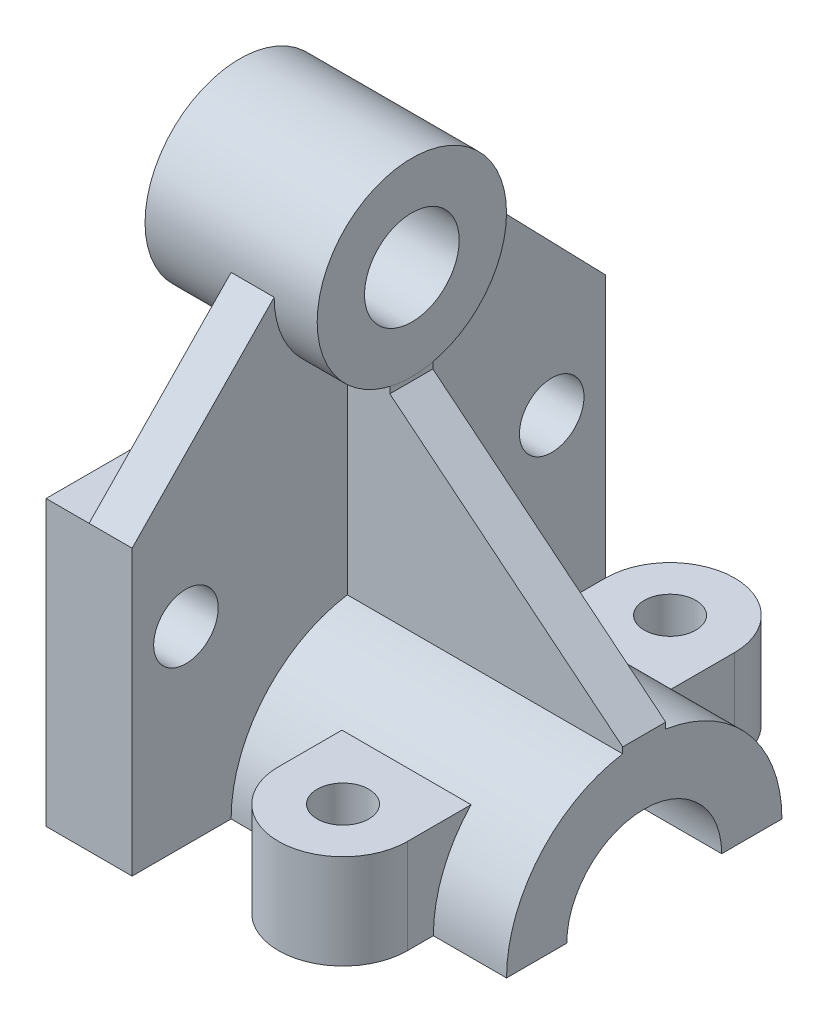
ISO-10303-21;
HEADER;
FILE_DESCRIPTION(('STEP AP214'),'2;1');
FILE_NAME('part.step','',(''),(''),'','','');
FILE_SCHEMA(('AUTOMOTIVE_DESIGN { 1 0 10303 214 1 1 1 1 }'));
ENDSEC;
DATA;
#1=APPLICATION_CONTEXT('core data for automotive mechanical design processes');
#2=APPLICATION_PROTOCOL_DEFINITION('international standard','automotive_design',2000,#1);
#3=PRODUCT_CONTEXT('',#1,'mechanical');
#4=PRODUCT('Part','Part','',(#3));
#5=PRODUCT_RELATED_PRODUCT_CATEGORY('part','',(#4));
#6=PRODUCT_DEFINITION_FORMATION('','',#4);
#7=PRODUCT_DEFINITION_CONTEXT('part definition',#1,'design');
#8=PRODUCT_DEFINITION('design','',#6,#7);
#9=PRODUCT_DEFINITION_SHAPE('','',#8);
#10=(LENGTH_UNIT() NAMED_UNIT(*) SI_UNIT(.MILLI.,.METRE.));
#11=(NAMED_UNIT(*) PLANE_ANGLE_UNIT() SI_UNIT($,.RADIAN.));
#12=(NAMED_UNIT(*) SI_UNIT($,.STERADIAN.) SOLID_ANGLE_UNIT());
#13=UNCERTAINTY_MEASURE_WITH_UNIT(LENGTH_MEASURE(1.E-05),#10,'distance_accuracy_value','');
#14=(GEOMETRIC_REPRESENTATION_CONTEXT(3) GLOBAL_UNCERTAINTY_ASSIGNED_CONTEXT((#13)) GLOBAL_UNIT_ASSIGNED_CONTEXT((#10,
#11,#12)) REPRESENTATION_CONTEXT('',''));
#15=CARTESIAN_POINT('',(0.,0.,0.));
#16=DIRECTION('',(0.,0.,1.));
#17=DIRECTION('',(1.,0.,0.));
#18=AXIS2_PLACEMENT_3D('',#15,#16,#17);
#19=CARTESIAN_POINT('',(10.,67.,0.));
#20=DIRECTION('',(1.,0.,0.));
#21=DIRECTION('',(0.,0.,-1.));
#22=AXIS2_PLACEMENT_3D('',#19,#20,#21);
#23=PLANE('',#22);
#24=CARTESIAN_POINT('',(10.,11.,-42.5));
#25=DIRECTION('',(1.,0.,0.));
#26=DIRECTION('',(0.,0.,-1.));
#27=AXIS2_PLACEMENT_3D('',#24,#25,#26);
#28=CIRCLE('',#27,7.5);
#29=CARTESIAN_POINT('',(10.,11.,-50.));
#30=VERTEX_POINT('',#29);
#31=EDGE_CURVE('E342',#30,#30,#28,.T.);
#32=ORIENTED_EDGE('',*,*,#31,.F.);
#33=EDGE_LOOP('',(#32));
#34=FACE_BOUND('',#33,.T.);
#35=DIRECTION('',(0.,-1.,0.));
#36=VECTOR('',#35,1.);
#37=CARTESIAN_POINT('',(10.,44.,-5.));
#38=LINE('',#37,#36);
#39=CARTESIAN_POINT('',(10.,45.5757147143715,-5.));
#40=VERTEX_POINT('',#39);
#41=CARTESIAN_POINT('',(10.,-1.39303874144178,-5.));
#42=VERTEX_POINT('',#41);
#43=EDGE_CURVE('E65',#40,#42,#38,.T.);
#44=ORIENTED_EDGE('',*,*,#43,.T.);
#45=CARTESIAN_POINT('',(10.,-33.,0.));
#46=DIRECTION('',(1.,0.,0.));
#47=DIRECTION('',(0.,0.,-1.));
#48=AXIS2_PLACEMENT_3D('',#45,#46,#47);
#49=CIRCLE('',#48,32.);
#50=CARTESIAN_POINT('',(10.,-33.,-32.));
#51=VERTEX_POINT('',#50);
#52=EDGE_CURVE('E314',#51,#42,#49,.T.);
#53=ORIENTED_EDGE('',*,*,#52,.F.);
#54=DIRECTION('',(0.,0.,-1.));
#55=VECTOR('',#54,1.);
#56=CARTESIAN_POINT('',(10.,-33.,55.));
#57=LINE('',#56,#55);
#58=CARTESIAN_POINT('',(10.,-33.,-55.));
#59=VERTEX_POINT('',#58);
#60=EDGE_CURVE('E354',#51,#59,#57,.T.);
#61=ORIENTED_EDGE('',*,*,#60,.T.);
#62=DIRECTION('',(0.,1.,0.));
#63=VECTOR('',#62,1.);
#64=CARTESIAN_POINT('',(10.,33.,-55.));
#65=LINE('',#64,#63);
#66=CARTESIAN_POINT('',(10.,33.,-55.));
#67=VERTEX_POINT('',#66);
#68=EDGE_CURVE('E350',#59,#67,#65,.T.);
#69=ORIENTED_EDGE('',*,*,#68,.T.);
#70=DIRECTION('',(0.,0.717580691628316,0.69647537716866));
#71=VECTOR('',#70,1.);
#72=CARTESIAN_POINT('',(10.,33.,-55.));
#73=LINE('',#72,#71);
#74=CARTESIAN_POINT('',(10.,67.,-22.));
#75=VERTEX_POINT('',#74);
#76=EDGE_CURVE('E391',#67,#75,#73,.T.);
#77=ORIENTED_EDGE('',*,*,#76,.T.);
#78=CARTESIAN_POINT('',(10.,67.,0.));
#79=DIRECTION('',(-1.,0.,0.));
#80=DIRECTION('',(0.,0.,-1.));
#81=AXIS2_PLACEMENT_3D('',#78,#79,#80);
#82=CIRCLE('',#81,22.);
#83=EDGE_CURVE('E414',#75,#40,#82,.T.);
#84=ORIENTED_EDGE('',*,*,#83,.T.);
#85=EDGE_LOOP('',(#44,#53,#61,#69,#77,#84));
#86=FACE_BOUND('',#85,.T.);
#87=ADVANCED_FACE('F39',(#34,#86),#23,.T.);
#88=CARTESIAN_POINT('',(10.,11.,42.5));
#89=DIRECTION('',(1.,0.,0.));
#90=DIRECTION('',(0.,0.,1.));
#91=AXIS2_PLACEMENT_3D('',#88,#89,#90);
#92=CIRCLE('',#91,7.5);
#93=CARTESIAN_POINT('',(10.,11.,50.));
#94=VERTEX_POINT('',#93);
#95=EDGE_CURVE('E341',#94,#94,#92,.T.);
#96=ORIENTED_EDGE('',*,*,#95,.F.);
#97=EDGE_LOOP('',(#96));
#98=FACE_BOUND('',#97,.T.);
#99=CARTESIAN_POINT('',(10.,-1.39303874144178,5.));
#100=VERTEX_POINT('',#99);
#101=CARTESIAN_POINT('',(10.,-33.,32.));
#102=VERTEX_POINT('',#101);
#103=EDGE_CURVE('E321',#100,#102,#49,.T.);
#104=ORIENTED_EDGE('',*,*,#103,.F.);
#105=DIRECTION('',(0.,-1.,0.));
#106=VECTOR('',#105,1.);
#107=CARTESIAN_POINT('',(10.,44.,5.));
#108=LINE('',#107,#106);
#109=CARTESIAN_POINT('',(10.,45.5757147143715,5.));
#110=VERTEX_POINT('',#109);
#111=EDGE_CURVE('E53',#110,#100,#108,.T.);
#112=ORIENTED_EDGE('',*,*,#111,.F.);
#113=CARTESIAN_POINT('',(10.,67.,22.));
#114=VERTEX_POINT('',#113);
#115=EDGE_CURVE('E413',#110,#114,#82,.T.);
#116=ORIENTED_EDGE('',*,*,#115,.T.);
#117=DIRECTION('',(0.,-0.717580691628316,0.69647537716866));
#118=VECTOR('',#117,1.);
#119=CARTESIAN_POINT('',(10.,67.,22.));
#120=LINE('',#119,#118);
#121=CARTESIAN_POINT('',(10.,33.,55.));
#122=VERTEX_POINT('',#121);
#123=EDGE_CURVE('E399',#114,#122,#120,.T.);
#124=ORIENTED_EDGE('',*,*,#123,.T.);
#125=DIRECTION('',(0.,-1.,0.));
#126=VECTOR('',#125,1.);
#127=CARTESIAN_POINT('',(10.,33.,55.));
#128=LINE('',#127,#126);
#129=CARTESIAN_POINT('',(10.,-33.,55.));
#130=VERTEX_POINT('',#129);
#131=EDGE_CURVE('E355',#122,#130,#128,.T.);
#132=ORIENTED_EDGE('',*,*,#131,.T.);
#133=EDGE_CURVE('E358',#130,#102,#57,.T.);
#134=ORIENTED_EDGE('',*,*,#133,.T.);
#135=EDGE_LOOP('',(#104,#112,#116,#124,#132,#134));
#136=FACE_BOUND('',#135,.T.);
#137=ADVANCED_FACE('F458',(#98,#136),#23,.T.);
#138=CARTESIAN_POINT('',(74.,-33.,0.));
#139=DIRECTION('',(-1.,0.,0.));
#140=DIRECTION('',(0.,0.,1.));
#141=AXIS2_PLACEMENT_3D('',#138,#139,#140);
#142=CYLINDRICAL_SURFACE('',#141,32.);
#143=DIRECTION('',(-1.,0.,0.));
#144=VECTOR('',#143,1.);
#145=CARTESIAN_POINT('',(74.,-1.39303874144178,-5.));
#146=LINE('',#145,#144);
#147=CARTESIAN_POINT('',(74.,-1.39303874144178,-5.));
#148=VERTEX_POINT('',#147);
#149=EDGE_CURVE('E238',#148,#42,#146,.T.);
#150=ORIENTED_EDGE('',*,*,#149,.F.);
#151=CARTESIAN_POINT('',(74.,-33.,0.));
#152=DIRECTION('',(1.,0.,0.));
#153=DIRECTION('',(0.,0.,-1.));
#154=AXIS2_PLACEMENT_3D('',#151,#152,#153);
#155=CIRCLE('',#154,32.);
#156=CARTESIAN_POINT('',(74.,-33.,-32.));
#157=VERTEX_POINT('',#156);
#158=EDGE_CURVE('E234',#157,#148,#155,.T.);
#159=ORIENTED_EDGE('',*,*,#158,.F.);
#160=DIRECTION('',(-1.,0.,0.));
#161=VECTOR('',#160,1.);
#162=CARTESIAN_POINT('',(74.,-33.,-32.));
#163=LINE('',#162,#161);
#164=CARTESIAN_POINT('',(57.,-33.,-32.));
#165=VERTEX_POINT('',#164);
#166=EDGE_CURVE('E335',#157,#165,#163,.T.);
#167=ORIENTED_EDGE('',*,*,#166,.T.);
#168=CARTESIAN_POINT('',(57.,-33.,0.));
#169=DIRECTION('',(1.,0.,0.));
#170=DIRECTION('',(0.,0.,-1.));
#171=AXIS2_PLACEMENT_3D('',#168,#169,#170);
#172=CIRCLE('',#171,32.);
#173=CARTESIAN_POINT('',(57.,-11.,-23.2379000772445));
#174=VERTEX_POINT('',#173);
#175=EDGE_CURVE('E382',#165,#174,#172,.T.);
#176=ORIENTED_EDGE('',*,*,#175,.T.);
#177=DIRECTION('',(-1.,0.,0.));
#178=VECTOR('',#177,1.);
#179=CARTESIAN_POINT('',(74.,-11.,-23.2379000772445));
#180=LINE('',#179,#178);
#181=CARTESIAN_POINT('',(27.,-11.,-23.2379000772445));
#182=VERTEX_POINT('',#181);
#183=EDGE_CURVE('E377',#182,#174,#180,.F.);
#184=ORIENTED_EDGE('',*,*,#183,.F.);
#185=CARTESIAN_POINT('',(27.,-33.,0.));
#186=DIRECTION('',(-1.,0.,0.));
#187=DIRECTION('',(0.,0.,1.));
#188=AXIS2_PLACEMENT_3D('',#185,#186,#187);
#189=CIRCLE('',#188,32.);
#190=CARTESIAN_POINT('',(27.,-33.,-32.));
#191=VERTEX_POINT('',#190);
#192=EDGE_CURVE('E384',#182,#191,#189,.T.);
#193=ORIENTED_EDGE('',*,*,#192,.T.);
#194=EDGE_CURVE('E331',#191,#51,#163,.T.);
#195=ORIENTED_EDGE('',*,*,#194,.T.);
#196=ORIENTED_EDGE('',*,*,#52,.T.);
#197=EDGE_LOOP('',(#150,#159,#167,#176,#184,#193,#195,#196));
#198=FACE_BOUND('',#197,.T.);
#199=ADVANCED_FACE('F463',(#198),#142,.T.);
#200=DIRECTION('',(-1.,0.,0.));
#201=VECTOR('',#200,1.);
#202=CARTESIAN_POINT('',(74.,-1.39303874144179,5.));
#203=LINE('',#202,#201);
#204=CARTESIAN_POINT('',(74.,-1.39303874144179,5.));
#205=VERTEX_POINT('',#204);
#206=EDGE_CURVE('E232',#100,#205,#203,.F.);
#207=ORIENTED_EDGE('',*,*,#206,.F.);
#208=ORIENTED_EDGE('',*,*,#103,.T.);
#209=DIRECTION('',(-1.,0.,0.));
#210=VECTOR('',#209,1.);
#211=CARTESIAN_POINT('',(74.,-33.,32.));
#212=LINE('',#211,#210);
#213=CARTESIAN_POINT('',(27.,-33.,32.));
#214=VERTEX_POINT('',#213);
#215=EDGE_CURVE('E329',#214,#102,#212,.T.);
#216=ORIENTED_EDGE('',*,*,#215,.F.);
#217=CARTESIAN_POINT('',(27.,-33.,0.));
#218=DIRECTION('',(-1.,0.,0.));
#219=DIRECTION('',(0.,0.,1.));
#220=AXIS2_PLACEMENT_3D('',#217,#218,#219);
#221=CIRCLE('',#220,32.);
#222=CARTESIAN_POINT('',(27.,-11.,23.2379000772445));
#223=VERTEX_POINT('',#222);
#224=EDGE_CURVE('E386',#214,#223,#221,.T.);
#225=ORIENTED_EDGE('',*,*,#224,.T.);
#226=DIRECTION('',(-1.,0.,0.));
#227=VECTOR('',#226,1.);
#228=CARTESIAN_POINT('',(74.,-11.,23.2379000772445));
#229=LINE('',#228,#227);
#230=CARTESIAN_POINT('',(57.,-11.,23.2379000772445));
#231=VERTEX_POINT('',#230);
#232=EDGE_CURVE('E387',#223,#231,#229,.F.);
#233=ORIENTED_EDGE('',*,*,#232,.T.);
#234=CARTESIAN_POINT('',(57.,-33.,0.));
#235=DIRECTION('',(1.,0.,0.));
#236=DIRECTION('',(0.,0.,-1.));
#237=AXIS2_PLACEMENT_3D('',#234,#235,#236);
#238=CIRCLE('',#237,32.);
#239=CARTESIAN_POINT('',(57.,-33.,32.));
#240=VERTEX_POINT('',#239);
#241=EDGE_CURVE('E394',#231,#240,#238,.T.);
#242=ORIENTED_EDGE('',*,*,#241,.T.);
#243=CARTESIAN_POINT('',(74.,-33.,32.));
#244=VERTEX_POINT('',#243);
#245=EDGE_CURVE('E327',#244,#240,#212,.T.);
#246=ORIENTED_EDGE('',*,*,#245,.F.);
#247=EDGE_CURVE('E320',#205,#244,#155,.T.);
#248=ORIENTED_EDGE('',*,*,#247,.F.);
#249=EDGE_LOOP('',(#207,#208,#216,#225,#233,#242,#246,#248));
#250=FACE_BOUND('',#249,.T.);
#251=ADVANCED_FACE('F516',(#250),#142,.T.);
#252=CARTESIAN_POINT('',(-20.,67.,0.));
#253=DIRECTION('',(1.,0.,0.));
#254=DIRECTION('',(0.,0.,-1.));
#255=AXIS2_PLACEMENT_3D('',#252,#253,#254);
#256=CYLINDRICAL_SURFACE('',#255,22.);
#257=CARTESIAN_POINT('',(-20.,67.,0.));
#258=DIRECTION('',(1.,0.,0.));
#259=DIRECTION('',(0.,0.,-1.));
#260=AXIS2_PLACEMENT_3D('',#257,#258,#259);
#261=CIRCLE('',#260,22.);
#262=CARTESIAN_POINT('',(-20.,67.,-22.));
#263=VERTEX_POINT('',#262);
#264=EDGE_CURVE('E11',#263,#263,#261,.T.);
#265=ORIENTED_EDGE('',*,*,#264,.T.);
#266=EDGE_LOOP('',(#265));
#267=FACE_BOUND('',#266,.T.);
#268=CARTESIAN_POINT('',(20.,67.,0.));
#269=DIRECTION('',(1.,0.,0.));
#270=DIRECTION('',(0.,0.,-1.));
#271=AXIS2_PLACEMENT_3D('',#268,#269,#270);
#272=CIRCLE('',#271,22.);
#273=CARTESIAN_POINT('',(20.,67.,-22.));
#274=VERTEX_POINT('',#273);
#275=EDGE_CURVE('E429',#274,#274,#272,.T.);
#276=ORIENTED_EDGE('',*,*,#275,.F.);
#277=EDGE_LOOP('',(#276));
#278=FACE_BOUND('',#277,.T.);
#279=CARTESIAN_POINT('',(19.8821035699118,67.,0.));
#280=DIRECTION('',(-1.,0.,0.));
#281=DIRECTION('',(0.,0.,1.));
#282=AXIS2_PLACEMENT_3D('',#279,#280,#281);
#283=CIRCLE('',#282,22.);
#284=CARTESIAN_POINT('',(19.8821035699118,45.5757147143715,5.));
#285=VERTEX_POINT('',#284);
#286=CARTESIAN_POINT('',(19.8821035699118,45.5757147143715,-5.));
#287=VERTEX_POINT('',#286);
#288=EDGE_CURVE('E255',#285,#287,#283,.F.);
#289=ORIENTED_EDGE('',*,*,#288,.T.);
#290=DIRECTION('',(1.,0.,0.));
#291=VECTOR('',#290,1.);
#292=CARTESIAN_POINT('',(-20.,45.5757147143715,-5.));
#293=LINE('',#292,#291);
#294=EDGE_CURVE('E248',#287,#40,#293,.F.);
#295=ORIENTED_EDGE('',*,*,#294,.T.);
#296=ORIENTED_EDGE('',*,*,#83,.F.);
#297=DIRECTION('',(1.,0.,0.));
#298=VECTOR('',#297,1.);
#299=CARTESIAN_POINT('',(0.,67.,-22.));
#300=LINE('',#299,#298);
#301=CARTESIAN_POINT('',(0.,67.,-22.));
#302=VERTEX_POINT('',#301);
#303=EDGE_CURVE('E422',#302,#75,#300,.T.);
#304=ORIENTED_EDGE('',*,*,#303,.F.);
#305=CARTESIAN_POINT('',(0.,67.,0.));
#306=DIRECTION('',(-1.,0.,0.));
#307=DIRECTION('',(0.,0.,-1.));
#308=AXIS2_PLACEMENT_3D('',#305,#306,#307);
#309=CIRCLE('',#308,22.);
#310=CARTESIAN_POINT('',(0.,67.,22.));
#311=VERTEX_POINT('',#310);
#312=EDGE_CURVE('E401',#302,#311,#309,.T.);
#313=ORIENTED_EDGE('',*,*,#312,.T.);
#314=DIRECTION('',(1.,0.,0.));
#315=VECTOR('',#314,1.);
#316=CARTESIAN_POINT('',(0.,67.,22.));
#317=LINE('',#316,#315);
#318=EDGE_CURVE('E417',#311,#114,#317,.T.);
#319=ORIENTED_EDGE('',*,*,#318,.T.);
#320=ORIENTED_EDGE('',*,*,#115,.F.);
#321=DIRECTION('',(1.,0.,0.));
#322=VECTOR('',#321,1.);
#323=CARTESIAN_POINT('',(-20.,45.5757147143715,5.));
#324=LINE('',#323,#322);
#325=EDGE_CURVE('E250',#110,#285,#324,.T.);
#326=ORIENTED_EDGE('',*,*,#325,.T.);
#327=EDGE_LOOP('',(#289,#295,#296,#304,#313,#319,#320,#326));
#328=FACE_BOUND('',#327,.T.);
#329=ADVANCED_FACE('F41',(#267,#278,#328),#256,.T.);
#330=CARTESIAN_POINT('',(-20.,67.,0.));
#331=DIRECTION('',(1.,0.,0.));
#332=DIRECTION('',(0.,0.,-1.));
#333=AXIS2_PLACEMENT_3D('',#330,#331,#332);
#334=PLANE('',#333);
#335=CARTESIAN_POINT('',(-20.,67.,0.));
#336=DIRECTION('',(1.,0.,0.));
#337=DIRECTION('',(0.,0.,-1.));
#338=AXIS2_PLACEMENT_3D('',#335,#336,#337);
#339=CIRCLE('',#338,11.);
#340=CARTESIAN_POINT('',(-20.,67.,-11.));
#341=VERTEX_POINT('',#340);
#342=EDGE_CURVE('E50',#341,#341,#339,.T.);
#343=ORIENTED_EDGE('',*,*,#342,.T.);
#344=EDGE_LOOP('',(#343));
#345=FACE_BOUND('',#344,.T.);
#346=ORIENTED_EDGE('',*,*,#264,.F.);
#347=EDGE_LOOP('',(#346));
#348=FACE_BOUND('',#347,.T.);
#349=ADVANCED_FACE('F432',(#345,#348),#334,.F.);
#350=CARTESIAN_POINT('',(-20.,67.,0.));
#351=DIRECTION('',(1.,0.,0.));
#352=DIRECTION('',(0.,0.,-1.));
#353=AXIS2_PLACEMENT_3D('',#350,#351,#352);
#354=CYLINDRICAL_SURFACE('',#353,11.);
#355=ORIENTED_EDGE('',*,*,#342,.F.);
#356=EDGE_LOOP('',(#355));
#357=FACE_BOUND('',#356,.T.);
#358=CARTESIAN_POINT('',(20.,67.,0.));
#359=DIRECTION('',(1.,0.,0.));
#360=DIRECTION('',(0.,0.,-1.));
#361=AXIS2_PLACEMENT_3D('',#358,#359,#360);
#362=CIRCLE('',#361,11.);
#363=CARTESIAN_POINT('',(20.,67.,-11.));
#364=VERTEX_POINT('',#363);
#365=EDGE_CURVE('E418',#364,#364,#362,.T.);
#366=ORIENTED_EDGE('',*,*,#365,.T.);
#367=EDGE_LOOP('',(#366));
#368=FACE_BOUND('',#367,.T.);
#369=ADVANCED_FACE('F440',(#357,#368),#354,.F.);
#370=CARTESIAN_POINT('',(20.,67.,0.));
#371=DIRECTION('',(1.,0.,0.));
#372=DIRECTION('',(0.,0.,-1.));
#373=AXIS2_PLACEMENT_3D('',#370,#371,#372);
#374=PLANE('',#373);
#375=ORIENTED_EDGE('',*,*,#275,.T.);
#376=EDGE_LOOP('',(#375));
#377=FACE_BOUND('',#376,.T.);
#378=ORIENTED_EDGE('',*,*,#365,.F.);
#379=EDGE_LOOP('',(#378));
#380=FACE_BOUND('',#379,.T.);
#381=ADVANCED_FACE('F439',(#377,#380),#374,.T.);
#382=CARTESIAN_POINT('',(0.,67.,22.));
#383=DIRECTION('',(0.,0.69647537716866,0.717580691628316));
#384=DIRECTION('',(0.,-0.717580691628316,0.69647537716866));
#385=AXIS2_PLACEMENT_3D('',#382,#383,#384);
#386=PLANE('',#385);
#387=ORIENTED_EDGE('',*,*,#123,.F.);
#388=ORIENTED_EDGE('',*,*,#318,.F.);
#389=DIRECTION('',(0.,-0.717580691628316,0.69647537716866));
#390=VECTOR('',#389,1.);
#391=CARTESIAN_POINT('',(0.,67.,22.));
#392=LINE('',#391,#390);
#393=CARTESIAN_POINT('',(0.,33.,55.));
#394=VERTEX_POINT('',#393);
#395=EDGE_CURVE('E403',#311,#394,#392,.T.);
#396=ORIENTED_EDGE('',*,*,#395,.T.);
#397=DIRECTION('',(1.,0.,0.));
#398=VECTOR('',#397,1.);
#399=CARTESIAN_POINT('',(0.,33.,55.));
#400=LINE('',#399,#398);
#401=EDGE_CURVE('E416',#394,#122,#400,.T.);
#402=ORIENTED_EDGE('',*,*,#401,.T.);
#403=EDGE_LOOP('',(#387,#388,#396,#402));
#404=FACE_BOUND('',#403,.T.);
#405=ADVANCED_FACE('F444',(#404),#386,.T.);
#406=CARTESIAN_POINT('',(0.,33.,-55.));
#407=DIRECTION('',(0.,0.69647537716866,-0.717580691628316));
#408=DIRECTION('',(0.,0.717580691628316,0.69647537716866));
#409=AXIS2_PLACEMENT_3D('',#406,#407,#408);
#410=PLANE('',#409);
#411=ORIENTED_EDGE('',*,*,#76,.F.);
#412=DIRECTION('',(1.,0.,0.));
#413=VECTOR('',#412,1.);
#414=CARTESIAN_POINT('',(0.,33.,-55.));
#415=LINE('',#414,#413);
#416=CARTESIAN_POINT('',(0.,33.,-55.));
#417=VERTEX_POINT('',#416);
#418=EDGE_CURVE('E409',#417,#67,#415,.T.);
#419=ORIENTED_EDGE('',*,*,#418,.F.);
#420=DIRECTION('',(0.,0.717580691628316,0.69647537716866));
#421=VECTOR('',#420,1.);
#422=CARTESIAN_POINT('',(0.,33.,-55.));
#423=LINE('',#422,#421);
#424=EDGE_CURVE('E397',#417,#302,#423,.T.);
#425=ORIENTED_EDGE('',*,*,#424,.T.);
#426=ORIENTED_EDGE('',*,*,#303,.T.);
#427=EDGE_LOOP('',(#411,#419,#425,#426));
#428=FACE_BOUND('',#427,.T.);
#429=ADVANCED_FACE('F452',(#428),#410,.T.);
#430=CARTESIAN_POINT('',(0.,67.,0.));
#431=DIRECTION('',(1.,0.,0.));
#432=DIRECTION('',(0.,0.,-1.));
#433=AXIS2_PLACEMENT_3D('',#430,#431,#432);
#434=PLANE('',#433);
#435=DIRECTION('',(0.,0.,-1.));
#436=VECTOR('',#435,1.);
#437=CARTESIAN_POINT('',(0.,33.,-55.));
#438=LINE('',#437,#436);
#439=EDGE_CURVE('E396',#394,#417,#438,.T.);
#440=ORIENTED_EDGE('',*,*,#439,.F.);
#441=ORIENTED_EDGE('',*,*,#395,.F.);
#442=ORIENTED_EDGE('',*,*,#312,.F.);
#443=ORIENTED_EDGE('',*,*,#424,.F.);
#444=EDGE_LOOP('',(#440,#441,#442,#443));
#445=FACE_BOUND('',#444,.T.);
#446=ADVANCED_FACE('F470',(#445),#434,.F.);
#447=CARTESIAN_POINT('',(10.,33.,55.));
#448=DIRECTION('',(0.,-1.,0.));
#449=DIRECTION('',(0.,0.,-1.));
#450=AXIS2_PLACEMENT_3D('',#447,#448,#449);
#451=PLANE('',#450);
#452=DIRECTION('',(-1.,0.,0.));
#453=VECTOR('',#452,1.);
#454=CARTESIAN_POINT('',(10.,33.,55.));
#455=LINE('',#454,#453);
#456=CARTESIAN_POINT('',(-10.,33.,55.));
#457=VERTEX_POINT('',#456);
#458=EDGE_CURVE('E372',#394,#457,#455,.T.);
#459=ORIENTED_EDGE('',*,*,#458,.F.);
#460=ORIENTED_EDGE('',*,*,#439,.T.);
#461=DIRECTION('',(-1.,0.,0.));
#462=VECTOR('',#461,1.);
#463=CARTESIAN_POINT('',(10.,33.,-55.));
#464=LINE('',#463,#462);
#465=CARTESIAN_POINT('',(-10.,33.,-55.));
#466=VERTEX_POINT('',#465);
#467=EDGE_CURVE('E376',#417,#466,#464,.T.);
#468=ORIENTED_EDGE('',*,*,#467,.T.);
#469=DIRECTION('',(0.,0.,1.));
#470=VECTOR('',#469,1.);
#471=CARTESIAN_POINT('',(-10.,33.,55.));
#472=LINE('',#471,#470);
#473=EDGE_CURVE('E361',#466,#457,#472,.T.);
#474=ORIENTED_EDGE('',*,*,#473,.T.);
#475=EDGE_LOOP('',(#459,#460,#468,#474));
#476=FACE_BOUND('',#475,.T.);
#477=ADVANCED_FACE('F471',(#476),#451,.F.);
#478=CARTESIAN_POINT('',(10.,0.,0.));
#479=DIRECTION('',(1.,0.,0.));
#480=DIRECTION('',(0.,0.,-1.));
#481=AXIS2_PLACEMENT_3D('',#478,#479,#480);
#482=PLANE('',#481);
#483=CARTESIAN_POINT('',(10.,-33.,0.));
#484=DIRECTION('',(-1.,0.,0.));
#485=DIRECTION('',(0.,0.,-1.));
#486=AXIS2_PLACEMENT_3D('',#483,#484,#485);
#487=CIRCLE('',#486,18.);
#488=CARTESIAN_POINT('',(10.,-33.,18.));
#489=VERTEX_POINT('',#488);
#490=CARTESIAN_POINT('',(10.,-33.,-18.));
#491=VERTEX_POINT('',#490);
#492=EDGE_CURVE('E307',#489,#491,#487,.T.);
#493=ORIENTED_EDGE('',*,*,#492,.F.);
#494=EDGE_CURVE('E359',#489,#491,#57,.T.);
#495=ORIENTED_EDGE('',*,*,#494,.T.);
#496=EDGE_LOOP('',(#493,#495));
#497=FACE_BOUND('',#496,.T.);
#498=ADVANCED_FACE('F532',(#497),#482,.T.);
#499=CARTESIAN_POINT('',(10.,33.,-55.));
#500=DIRECTION('',(0.,0.,1.));
#501=DIRECTION('',(0.,-1.,0.));
#502=AXIS2_PLACEMENT_3D('',#499,#500,#501);
#503=PLANE('',#502);
#504=DIRECTION('',(0.,1.,0.));
#505=VECTOR('',#504,1.);
#506=CARTESIAN_POINT('',(-10.,33.,-55.));
#507=LINE('',#506,#505);
#508=CARTESIAN_POINT('',(-10.,-33.,-55.));
#509=VERTEX_POINT('',#508);
#510=EDGE_CURVE('E338',#509,#466,#507,.T.);
#511=ORIENTED_EDGE('',*,*,#510,.T.);
#512=ORIENTED_EDGE('',*,*,#467,.F.);
#513=ORIENTED_EDGE('',*,*,#418,.T.);
#514=ORIENTED_EDGE('',*,*,#68,.F.);
#515=DIRECTION('',(-1.,0.,0.));
#516=VECTOR('',#515,1.);
#517=CARTESIAN_POINT('',(10.,-33.,-55.));
#518=LINE('',#517,#516);
#519=EDGE_CURVE('E360',#59,#509,#518,.T.);
#520=ORIENTED_EDGE('',*,*,#519,.T.);
#521=EDGE_LOOP('',(#511,#512,#513,#514,#520));
#522=FACE_BOUND('',#521,.T.);
#523=ADVANCED_FACE('F485',(#522),#503,.F.);
#524=CARTESIAN_POINT('',(10.,33.,55.));
#525=DIRECTION('',(0.,0.,-1.));
#526=DIRECTION('',(0.,1.,0.));
#527=AXIS2_PLACEMENT_3D('',#524,#525,#526);
#528=PLANE('',#527);
#529=DIRECTION('',(0.,-1.,0.));
#530=VECTOR('',#529,1.);
#531=CARTESIAN_POINT('',(-10.,33.,55.));
#532=LINE('',#531,#530);
#533=CARTESIAN_POINT('',(-10.,-33.,55.));
#534=VERTEX_POINT('',#533);
#535=EDGE_CURVE('E366',#457,#534,#532,.T.);
#536=ORIENTED_EDGE('',*,*,#535,.T.);
#537=DIRECTION('',(-1.,0.,0.));
#538=VECTOR('',#537,1.);
#539=CARTESIAN_POINT('',(10.,-33.,55.));
#540=LINE('',#539,#538);
#541=EDGE_CURVE('E371',#130,#534,#540,.T.);
#542=ORIENTED_EDGE('',*,*,#541,.F.);
#543=ORIENTED_EDGE('',*,*,#131,.F.);
#544=ORIENTED_EDGE('',*,*,#401,.F.);
#545=ORIENTED_EDGE('',*,*,#458,.T.);
#546=EDGE_LOOP('',(#536,#542,#543,#544,#545));
#547=FACE_BOUND('',#546,.T.);
#548=ADVANCED_FACE('F491',(#547),#528,.F.);
#549=CARTESIAN_POINT('',(10.,-33.,55.));
#550=DIRECTION('',(0.,1.,0.));
#551=DIRECTION('',(0.,0.,1.));
#552=AXIS2_PLACEMENT_3D('',#549,#550,#551);
#553=PLANE('',#552);
#554=CARTESIAN_POINT('',(42.,-33.,-38.));
#555=DIRECTION('',(0.,1.,0.));
#556=DIRECTION('',(0.,0.,1.));
#557=AXIS2_PLACEMENT_3D('',#554,#555,#556);
#558=CIRCLE('',#557,6.);
#559=CARTESIAN_POINT('',(42.,-33.,-32.));
#560=VERTEX_POINT('',#559);
#561=EDGE_CURVE('E259',#560,#560,#558,.T.);
#562=ORIENTED_EDGE('',*,*,#561,.T.);
#563=EDGE_LOOP('',(#562));
#564=FACE_BOUND('',#563,.T.);
#565=CARTESIAN_POINT('',(42.,-33.,38.));
#566=DIRECTION('',(0.,1.,0.));
#567=DIRECTION('',(0.,0.,1.));
#568=AXIS2_PLACEMENT_3D('',#565,#566,#567);
#569=CIRCLE('',#568,6.);
#570=CARTESIAN_POINT('',(42.,-33.,44.));
#571=VERTEX_POINT('',#570);
#572=EDGE_CURVE('E226',#571,#571,#569,.T.);
#573=ORIENTED_EDGE('',*,*,#572,.T.);
#574=EDGE_LOOP('',(#573));
#575=FACE_BOUND('',#574,.T.);
#576=ORIENTED_EDGE('',*,*,#494,.F.);
#577=DIRECTION('',(-1.,0.,0.));
#578=VECTOR('',#577,1.);
#579=CARTESIAN_POINT('',(74.,-33.,18.));
#580=LINE('',#579,#578);
#581=CARTESIAN_POINT('',(74.,-33.,18.));
#582=VERTEX_POINT('',#581);
#583=EDGE_CURVE('E322',#582,#489,#580,.T.);
#584=ORIENTED_EDGE('',*,*,#583,.F.);
#585=DIRECTION('',(0.,0.,-1.));
#586=VECTOR('',#585,1.);
#587=CARTESIAN_POINT('',(74.,-33.,32.));
#588=LINE('',#587,#586);
#589=EDGE_CURVE('E316',#244,#582,#588,.T.);
#590=ORIENTED_EDGE('',*,*,#589,.F.);
#591=ORIENTED_EDGE('',*,*,#245,.T.);
#592=DIRECTION('',(0.,0.,1.));
#593=VECTOR('',#592,1.);
#594=CARTESIAN_POINT('',(57.,-33.,18.));
#595=LINE('',#594,#593);
#596=CARTESIAN_POINT('',(57.,-33.,38.));
#597=VERTEX_POINT('',#596);
#598=EDGE_CURVE('E273',#240,#597,#595,.T.);
#599=ORIENTED_EDGE('',*,*,#598,.T.);
#600=CARTESIAN_POINT('',(42.,-33.,38.));
#601=DIRECTION('',(0.,-1.,0.));
#602=DIRECTION('',(0.,0.,1.));
#603=AXIS2_PLACEMENT_3D('',#600,#601,#602);
#604=CIRCLE('',#603,15.);
#605=CARTESIAN_POINT('',(27.,-33.,38.));
#606=VERTEX_POINT('',#605);
#607=EDGE_CURVE('E278',#597,#606,#604,.T.);
#608=ORIENTED_EDGE('',*,*,#607,.T.);
#609=DIRECTION('',(0.,0.,-1.));
#610=VECTOR('',#609,1.);
#611=CARTESIAN_POINT('',(27.,-33.,38.));
#612=LINE('',#611,#610);
#613=EDGE_CURVE('E280',#606,#214,#612,.T.);
#614=ORIENTED_EDGE('',*,*,#613,.T.);
#615=ORIENTED_EDGE('',*,*,#215,.T.);
#616=ORIENTED_EDGE('',*,*,#133,.F.);
#617=ORIENTED_EDGE('',*,*,#541,.T.);
#618=DIRECTION('',(0.,0.,-1.));
#619=VECTOR('',#618,1.);
#620=CARTESIAN_POINT('',(-10.,-33.,55.));
#621=LINE('',#620,#619);
#622=EDGE_CURVE('E353',#534,#509,#621,.T.);
#623=ORIENTED_EDGE('',*,*,#622,.T.);
#624=ORIENTED_EDGE('',*,*,#519,.F.);
#625=ORIENTED_EDGE('',*,*,#60,.F.);
#626=ORIENTED_EDGE('',*,*,#194,.F.);
#627=DIRECTION('',(0.,0.,-1.));
#628=VECTOR('',#627,1.);
#629=CARTESIAN_POINT('',(27.,-33.,-38.));
#630=LINE('',#629,#628);
#631=CARTESIAN_POINT('',(27.,-33.,-38.));
#632=VERTEX_POINT('',#631);
#633=EDGE_CURVE('E295',#191,#632,#630,.T.);
#634=ORIENTED_EDGE('',*,*,#633,.T.);
#635=CARTESIAN_POINT('',(42.,-33.,-38.));
#636=DIRECTION('',(0.,-1.,0.));
#637=DIRECTION('',(0.,0.,-1.));
#638=AXIS2_PLACEMENT_3D('',#635,#636,#637);
#639=CIRCLE('',#638,15.);
#640=CARTESIAN_POINT('',(57.,-33.,-38.));
#641=VERTEX_POINT('',#640);
#642=EDGE_CURVE('E282',#632,#641,#639,.T.);
#643=ORIENTED_EDGE('',*,*,#642,.T.);
#644=DIRECTION('',(0.,0.,1.));
#645=VECTOR('',#644,1.);
#646=CARTESIAN_POINT('',(57.,-33.,-18.));
#647=LINE('',#646,#645);
#648=EDGE_CURVE('E305',#641,#165,#647,.T.);
#649=ORIENTED_EDGE('',*,*,#648,.T.);
#650=ORIENTED_EDGE('',*,*,#166,.F.);
#651=DIRECTION('',(0.,0.,-1.));
#652=VECTOR('',#651,1.);
#653=CARTESIAN_POINT('',(74.,-33.,-18.));
#654=LINE('',#653,#652);
#655=CARTESIAN_POINT('',(74.,-33.,-18.));
#656=VERTEX_POINT('',#655);
#657=EDGE_CURVE('E313',#656,#157,#654,.T.);
#658=ORIENTED_EDGE('',*,*,#657,.F.);
#659=DIRECTION('',(-1.,0.,0.));
#660=VECTOR('',#659,1.);
#661=CARTESIAN_POINT('',(74.,-33.,-18.));
#662=LINE('',#661,#660);
#663=EDGE_CURVE('E332',#656,#491,#662,.T.);
#664=ORIENTED_EDGE('',*,*,#663,.T.);
#665=EDGE_LOOP('',(#576,#584,#590,#591,#599,#608,#614,#615,#616,#617,#623,#624,#625,#626,#634,
#643,#649,#650,#658,#664));
#666=FACE_BOUND('',#665,.T.);
#667=ADVANCED_FACE('F497',(#564,#575,#666),#553,.F.);
#668=CARTESIAN_POINT('',(-10.,0.,0.));
#669=DIRECTION('',(1.,0.,0.));
#670=DIRECTION('',(0.,0.,-1.));
#671=AXIS2_PLACEMENT_3D('',#668,#669,#670);
#672=PLANE('',#671);
#673=CARTESIAN_POINT('',(-10.,11.,-42.5));
#674=DIRECTION('',(1.,0.,0.));
#675=DIRECTION('',(0.,0.,-1.));
#676=AXIS2_PLACEMENT_3D('',#673,#674,#675);
#677=CIRCLE('',#676,7.5);
#678=CARTESIAN_POINT('',(-10.,11.,-50.));
#679=VERTEX_POINT('',#678);
#680=EDGE_CURVE('E340',#679,#679,#677,.T.);
#681=ORIENTED_EDGE('',*,*,#680,.T.);
#682=EDGE_LOOP('',(#681));
#683=FACE_BOUND('',#682,.T.);
#684=CARTESIAN_POINT('',(-10.,11.,42.5));
#685=DIRECTION('',(1.,0.,0.));
#686=DIRECTION('',(0.,0.,1.));
#687=AXIS2_PLACEMENT_3D('',#684,#685,#686);
#688=CIRCLE('',#687,7.5);
#689=CARTESIAN_POINT('',(-10.,11.,50.));
#690=VERTEX_POINT('',#689);
#691=EDGE_CURVE('E337',#690,#690,#688,.T.);
#692=ORIENTED_EDGE('',*,*,#691,.T.);
#693=EDGE_LOOP('',(#692));
#694=FACE_BOUND('',#693,.T.);
#695=ORIENTED_EDGE('',*,*,#510,.F.);
#696=ORIENTED_EDGE('',*,*,#622,.F.);
#697=ORIENTED_EDGE('',*,*,#535,.F.);
#698=ORIENTED_EDGE('',*,*,#473,.F.);
#699=EDGE_LOOP('',(#695,#696,#697,#698));
#700=FACE_BOUND('',#699,.T.);
#701=ADVANCED_FACE('F490',(#683,#694,#700),#672,.F.);
#702=CARTESIAN_POINT('',(-10.,11.,42.5));
#703=DIRECTION('',(1.,0.,0.));
#704=DIRECTION('',(0.,0.,-1.));
#705=AXIS2_PLACEMENT_3D('',#702,#703,#704);
#706=CYLINDRICAL_SURFACE('',#705,7.5);
#707=ORIENTED_EDGE('',*,*,#691,.F.);
#708=EDGE_LOOP('',(#707));
#709=FACE_BOUND('',#708,.T.);
#710=ORIENTED_EDGE('',*,*,#95,.T.);
#711=EDGE_LOOP('',(#710));
#712=FACE_BOUND('',#711,.T.);
#713=ADVANCED_FACE('F543',(#709,#712),#706,.F.);
#714=CARTESIAN_POINT('',(-10.,11.,-42.5));
#715=DIRECTION('',(1.,0.,0.));
#716=DIRECTION('',(0.,0.,-1.));
#717=AXIS2_PLACEMENT_3D('',#714,#715,#716);
#718=CYLINDRICAL_SURFACE('',#717,7.5);
#719=ORIENTED_EDGE('',*,*,#680,.F.);
#720=EDGE_LOOP('',(#719));
#721=FACE_BOUND('',#720,.T.);
#722=ORIENTED_EDGE('',*,*,#31,.T.);
#723=EDGE_LOOP('',(#722));
#724=FACE_BOUND('',#723,.T.);
#725=ADVANCED_FACE('F568',(#721,#724),#718,.F.);
#726=CARTESIAN_POINT('',(74.,-33.,0.));
#727=DIRECTION('',(-1.,0.,0.));
#728=DIRECTION('',(0.,0.,1.));
#729=AXIS2_PLACEMENT_3D('',#726,#727,#728);
#730=CYLINDRICAL_SURFACE('',#729,18.);
#731=ORIENTED_EDGE('',*,*,#492,.T.);
#732=ORIENTED_EDGE('',*,*,#663,.F.);
#733=CARTESIAN_POINT('',(74.,-33.,0.));
#734=DIRECTION('',(-1.,0.,0.));
#735=DIRECTION('',(0.,0.,-1.));
#736=AXIS2_PLACEMENT_3D('',#733,#734,#735);
#737=CIRCLE('',#736,18.);
#738=EDGE_CURVE('E311',#582,#656,#737,.T.);
#739=ORIENTED_EDGE('',*,*,#738,.F.);
#740=ORIENTED_EDGE('',*,*,#583,.T.);
#741=EDGE_LOOP('',(#731,#732,#739,#740));
#742=FACE_BOUND('',#741,.T.);
#743=ADVANCED_FACE('F521',(#742),#730,.F.);
#744=CARTESIAN_POINT('',(74.,-33.,0.));
#745=DIRECTION('',(1.,0.,0.));
#746=DIRECTION('',(0.,0.,-1.));
#747=AXIS2_PLACEMENT_3D('',#744,#745,#746);
#748=PLANE('',#747);
#749=ORIENTED_EDGE('',*,*,#158,.T.);
#750=DIRECTION('',(0.,1.,0.));
#751=VECTOR('',#750,1.);
#752=CARTESIAN_POINT('',(74.,-2.,-5.));
#753=LINE('',#752,#751);
#754=CARTESIAN_POINT('',(74.,0.,-5.));
#755=VERTEX_POINT('',#754);
#756=EDGE_CURVE('E214',#148,#755,#753,.T.);
#757=ORIENTED_EDGE('',*,*,#756,.T.);
#758=DIRECTION('',(0.,0.,-1.));
#759=VECTOR('',#758,1.);
#760=CARTESIAN_POINT('',(74.,0.,5.));
#761=LINE('',#760,#759);
#762=CARTESIAN_POINT('',(74.,0.,5.));
#763=VERTEX_POINT('',#762);
#764=EDGE_CURVE('E225',#763,#755,#761,.T.);
#765=ORIENTED_EDGE('',*,*,#764,.F.);
#766=DIRECTION('',(0.,1.,0.));
#767=VECTOR('',#766,1.);
#768=CARTESIAN_POINT('',(74.,-2.,5.));
#769=LINE('',#768,#767);
#770=EDGE_CURVE('E236',#205,#763,#769,.T.);
#771=ORIENTED_EDGE('',*,*,#770,.F.);
#772=ORIENTED_EDGE('',*,*,#247,.T.);
#773=ORIENTED_EDGE('',*,*,#589,.T.);
#774=ORIENTED_EDGE('',*,*,#738,.T.);
#775=ORIENTED_EDGE('',*,*,#657,.T.);
#776=EDGE_LOOP('',(#749,#757,#765,#771,#772,#773,#774,#775));
#777=FACE_BOUND('',#776,.T.);
#778=ADVANCED_FACE('F235',(#777),#748,.T.);
#779=CARTESIAN_POINT('',(42.,-11.,-38.));
#780=DIRECTION('',(0.,-1.,0.));
#781=DIRECTION('',(0.,0.,-1.));
#782=AXIS2_PLACEMENT_3D('',#779,#780,#781);
#783=PLANE('',#782);
#784=CARTESIAN_POINT('',(42.,-11.,-38.));
#785=DIRECTION('',(0.,1.,0.));
#786=DIRECTION('',(0.,0.,1.));
#787=AXIS2_PLACEMENT_3D('',#784,#785,#786);
#788=CIRCLE('',#787,6.);
#789=CARTESIAN_POINT('',(42.,-11.,-32.));
#790=VERTEX_POINT('',#789);
#791=EDGE_CURVE('E264',#790,#790,#788,.T.);
#792=ORIENTED_EDGE('',*,*,#791,.F.);
#793=EDGE_LOOP('',(#792));
#794=FACE_BOUND('',#793,.T.);
#795=DIRECTION('',(0.,0.,-1.));
#796=VECTOR('',#795,1.);
#797=CARTESIAN_POINT('',(27.,-11.,-38.));
#798=LINE('',#797,#796);
#799=CARTESIAN_POINT('',(27.,-11.,-38.));
#800=VERTEX_POINT('',#799);
#801=EDGE_CURVE('E300',#182,#800,#798,.T.);
#802=ORIENTED_EDGE('',*,*,#801,.F.);
#803=ORIENTED_EDGE('',*,*,#183,.T.);
#804=DIRECTION('',(0.,0.,1.));
#805=VECTOR('',#804,1.);
#806=CARTESIAN_POINT('',(57.,-11.,-18.));
#807=LINE('',#806,#805);
#808=CARTESIAN_POINT('',(57.,-11.,-38.));
#809=VERTEX_POINT('',#808);
#810=EDGE_CURVE('E291',#809,#174,#807,.T.);
#811=ORIENTED_EDGE('',*,*,#810,.F.);
#812=CARTESIAN_POINT('',(42.,-11.,-38.));
#813=DIRECTION('',(0.,-1.,0.));
#814=DIRECTION('',(0.,0.,-1.));
#815=AXIS2_PLACEMENT_3D('',#812,#813,#814);
#816=CIRCLE('',#815,15.);
#817=EDGE_CURVE('E289',#800,#809,#816,.T.);
#818=ORIENTED_EDGE('',*,*,#817,.F.);
#819=EDGE_LOOP('',(#802,#803,#811,#818));
#820=FACE_BOUND('',#819,.T.);
#821=ADVANCED_FACE('F583',(#794,#820),#783,.F.);
#822=CARTESIAN_POINT('',(42.,-11.,-38.));
#823=DIRECTION('',(0.,-1.,0.));
#824=DIRECTION('',(0.,0.,-1.));
#825=AXIS2_PLACEMENT_3D('',#822,#823,#824);
#826=CYLINDRICAL_SURFACE('',#825,15.);
#827=ORIENTED_EDGE('',*,*,#642,.F.);
#828=DIRECTION('',(0.,-1.,0.));
#829=VECTOR('',#828,1.);
#830=CARTESIAN_POINT('',(27.,-11.,-38.));
#831=LINE('',#830,#829);
#832=EDGE_CURVE('E306',#800,#632,#831,.T.);
#833=ORIENTED_EDGE('',*,*,#832,.F.);
#834=ORIENTED_EDGE('',*,*,#817,.T.);
#835=DIRECTION('',(0.,-1.,0.));
#836=VECTOR('',#835,1.);
#837=CARTESIAN_POINT('',(57.,-11.,-38.));
#838=LINE('',#837,#836);
#839=EDGE_CURVE('E299',#809,#641,#838,.T.);
#840=ORIENTED_EDGE('',*,*,#839,.T.);
#841=EDGE_LOOP('',(#827,#833,#834,#840));
#842=FACE_BOUND('',#841,.T.);
#843=ADVANCED_FACE('F590',(#842),#826,.T.);
#844=CARTESIAN_POINT('',(27.,-11.,-38.));
#845=DIRECTION('',(-1.,0.,0.));
#846=DIRECTION('',(0.,0.,1.));
#847=AXIS2_PLACEMENT_3D('',#844,#845,#846);
#848=PLANE('',#847);
#849=ORIENTED_EDGE('',*,*,#192,.F.);
#850=ORIENTED_EDGE('',*,*,#801,.T.);
#851=ORIENTED_EDGE('',*,*,#832,.T.);
#852=ORIENTED_EDGE('',*,*,#633,.F.);
#853=EDGE_LOOP('',(#849,#850,#851,#852));
#854=FACE_BOUND('',#853,.T.);
#855=ADVANCED_FACE('F600',(#854),#848,.T.);
#856=CARTESIAN_POINT('',(57.,-11.,-18.));
#857=DIRECTION('',(1.,0.,0.));
#858=DIRECTION('',(0.,0.,-1.));
#859=AXIS2_PLACEMENT_3D('',#856,#857,#858);
#860=PLANE('',#859);
#861=ORIENTED_EDGE('',*,*,#175,.F.);
#862=ORIENTED_EDGE('',*,*,#648,.F.);
#863=ORIENTED_EDGE('',*,*,#839,.F.);
#864=ORIENTED_EDGE('',*,*,#810,.T.);
#865=EDGE_LOOP('',(#861,#862,#863,#864));
#866=FACE_BOUND('',#865,.T.);
#867=ADVANCED_FACE('F603',(#866),#860,.T.);
#868=CARTESIAN_POINT('',(42.,-11.,38.));
#869=DIRECTION('',(0.,1.,0.));
#870=DIRECTION('',(0.,0.,1.));
#871=AXIS2_PLACEMENT_3D('',#868,#869,#870);
#872=PLANE('',#871);
#873=CARTESIAN_POINT('',(42.,-11.,38.));
#874=DIRECTION('',(0.,1.,0.));
#875=DIRECTION('',(0.,0.,1.));
#876=AXIS2_PLACEMENT_3D('',#873,#874,#875);
#877=CIRCLE('',#876,6.);
#878=CARTESIAN_POINT('',(42.,-11.,44.));
#879=VERTEX_POINT('',#878);
#880=EDGE_CURVE('E261',#879,#879,#877,.T.);
#881=ORIENTED_EDGE('',*,*,#880,.F.);
#882=EDGE_LOOP('',(#881));
#883=FACE_BOUND('',#882,.T.);
#884=ORIENTED_EDGE('',*,*,#232,.F.);
#885=DIRECTION('',(0.,0.,-1.));
#886=VECTOR('',#885,1.);
#887=CARTESIAN_POINT('',(27.,-11.,38.));
#888=LINE('',#887,#886);
#889=CARTESIAN_POINT('',(27.,-11.,38.));
#890=VERTEX_POINT('',#889);
#891=EDGE_CURVE('E281',#890,#223,#888,.T.);
#892=ORIENTED_EDGE('',*,*,#891,.F.);
#893=CARTESIAN_POINT('',(42.,-11.,38.));
#894=DIRECTION('',(0.,-1.,0.));
#895=DIRECTION('',(0.,0.,1.));
#896=AXIS2_PLACEMENT_3D('',#893,#894,#895);
#897=CIRCLE('',#896,15.);
#898=CARTESIAN_POINT('',(57.,-11.,38.));
#899=VERTEX_POINT('',#898);
#900=EDGE_CURVE('E279',#899,#890,#897,.T.);
#901=ORIENTED_EDGE('',*,*,#900,.F.);
#902=DIRECTION('',(0.,0.,1.));
#903=VECTOR('',#902,1.);
#904=CARTESIAN_POINT('',(57.,-11.,18.));
#905=LINE('',#904,#903);
#906=EDGE_CURVE('E275',#231,#899,#905,.T.);
#907=ORIENTED_EDGE('',*,*,#906,.F.);
#908=EDGE_LOOP('',(#884,#892,#901,#907));
#909=FACE_BOUND('',#908,.T.);
#910=ADVANCED_FACE('F613',(#883,#909),#872,.T.);
#911=CARTESIAN_POINT('',(42.,-11.,38.));
#912=DIRECTION('',(0.,-1.,0.));
#913=DIRECTION('',(0.,0.,-1.));
#914=AXIS2_PLACEMENT_3D('',#911,#912,#913);
#915=CYLINDRICAL_SURFACE('',#914,15.);
#916=ORIENTED_EDGE('',*,*,#607,.F.);
#917=DIRECTION('',(0.,-1.,0.));
#918=VECTOR('',#917,1.);
#919=CARTESIAN_POINT('',(57.,-11.,38.));
#920=LINE('',#919,#918);
#921=EDGE_CURVE('E263',#899,#597,#920,.T.);
#922=ORIENTED_EDGE('',*,*,#921,.F.);
#923=ORIENTED_EDGE('',*,*,#900,.T.);
#924=DIRECTION('',(0.,-1.,0.));
#925=VECTOR('',#924,1.);
#926=CARTESIAN_POINT('',(27.,-11.,38.));
#927=LINE('',#926,#925);
#928=EDGE_CURVE('E269',#890,#606,#927,.T.);
#929=ORIENTED_EDGE('',*,*,#928,.T.);
#930=EDGE_LOOP('',(#916,#922,#923,#929));
#931=FACE_BOUND('',#930,.T.);
#932=ADVANCED_FACE('F623',(#931),#915,.T.);
#933=CARTESIAN_POINT('',(57.,-11.,18.));
#934=DIRECTION('',(1.,0.,0.));
#935=DIRECTION('',(0.,0.,-1.));
#936=AXIS2_PLACEMENT_3D('',#933,#934,#935);
#937=PLANE('',#936);
#938=ORIENTED_EDGE('',*,*,#241,.F.);
#939=ORIENTED_EDGE('',*,*,#906,.T.);
#940=ORIENTED_EDGE('',*,*,#921,.T.);
#941=ORIENTED_EDGE('',*,*,#598,.F.);
#942=EDGE_LOOP('',(#938,#939,#940,#941));
#943=FACE_BOUND('',#942,.T.);
#944=ADVANCED_FACE('F627',(#943),#937,.T.);
#945=CARTESIAN_POINT('',(27.,-11.,38.));
#946=DIRECTION('',(-1.,0.,0.));
#947=DIRECTION('',(0.,0.,1.));
#948=AXIS2_PLACEMENT_3D('',#945,#946,#947);
#949=PLANE('',#948);
#950=ORIENTED_EDGE('',*,*,#224,.F.);
#951=ORIENTED_EDGE('',*,*,#613,.F.);
#952=ORIENTED_EDGE('',*,*,#928,.F.);
#953=ORIENTED_EDGE('',*,*,#891,.T.);
#954=EDGE_LOOP('',(#950,#951,#952,#953));
#955=FACE_BOUND('',#954,.T.);
#956=ADVANCED_FACE('F640',(#955),#949,.T.);
#957=CARTESIAN_POINT('',(42.,-33.,38.));
#958=DIRECTION('',(0.,1.,0.));
#959=DIRECTION('',(0.,0.,1.));
#960=AXIS2_PLACEMENT_3D('',#957,#958,#959);
#961=CYLINDRICAL_SURFACE('',#960,6.);
#962=ORIENTED_EDGE('',*,*,#572,.F.);
#963=EDGE_LOOP('',(#962));
#964=FACE_BOUND('',#963,.T.);
#965=ORIENTED_EDGE('',*,*,#880,.T.);
#966=EDGE_LOOP('',(#965));
#967=FACE_BOUND('',#966,.T.);
#968=ADVANCED_FACE('F643',(#964,#967),#961,.F.);
#969=CARTESIAN_POINT('',(42.,-33.,-38.));
#970=DIRECTION('',(0.,1.,0.));
#971=DIRECTION('',(0.,0.,1.));
#972=AXIS2_PLACEMENT_3D('',#969,#970,#971);
#973=CYLINDRICAL_SURFACE('',#972,6.);
#974=ORIENTED_EDGE('',*,*,#561,.F.);
#975=EDGE_LOOP('',(#974));
#976=FACE_BOUND('',#975,.T.);
#977=ORIENTED_EDGE('',*,*,#791,.T.);
#978=EDGE_LOOP('',(#977));
#979=FACE_BOUND('',#978,.T.);
#980=ADVANCED_FACE('F652',(#976,#979),#973,.F.);
#981=CARTESIAN_POINT('',(74.,0.,5.));
#982=DIRECTION('',(-0.630844846822868,-0.775909001904883,0.));
#983=DIRECTION('',(0.775909001904883,-0.630844846822868,0.));
#984=AXIS2_PLACEMENT_3D('',#981,#982,#983);
#985=PLANE('',#984);
#986=DIRECTION('',(-0.775909001904883,0.630844846822868,0.));
#987=VECTOR('',#986,1.);
#988=CARTESIAN_POINT('',(74.,0.,-5.));
#989=LINE('',#988,#987);
#990=CARTESIAN_POINT('',(19.8821035699118,44.,-5.));
#991=VERTEX_POINT('',#990);
#992=EDGE_CURVE('E206',#755,#991,#989,.T.);
#993=ORIENTED_EDGE('',*,*,#992,.T.);
#994=DIRECTION('',(0.,0.,-1.));
#995=VECTOR('',#994,1.);
#996=CARTESIAN_POINT('',(19.8821035699118,44.,5.));
#997=LINE('',#996,#995);
#998=CARTESIAN_POINT('',(19.8821035699118,44.,5.));
#999=VERTEX_POINT('',#998);
#1000=EDGE_CURVE('E230',#999,#991,#997,.T.);
#1001=ORIENTED_EDGE('',*,*,#1000,.F.);
#1002=DIRECTION('',(-0.775909001904883,0.630844846822868,0.));
#1003=VECTOR('',#1002,1.);
#1004=CARTESIAN_POINT('',(74.,0.,5.));
#1005=LINE('',#1004,#1003);
#1006=EDGE_CURVE('E222',#763,#999,#1005,.T.);
#1007=ORIENTED_EDGE('',*,*,#1006,.F.);
#1008=ORIENTED_EDGE('',*,*,#764,.T.);
#1009=EDGE_LOOP('',(#993,#1001,#1007,#1008));
#1010=FACE_BOUND('',#1009,.T.);
#1011=ADVANCED_FACE('F223',(#1010),#985,.F.);
#1012=CARTESIAN_POINT('',(0.,0.,5.));
#1013=DIRECTION('',(0.,0.,1.));
#1014=DIRECTION('',(1.,0.,0.));
#1015=AXIS2_PLACEMENT_3D('',#1012,#1013,#1014);
#1016=PLANE('',#1015);
#1017=ORIENTED_EDGE('',*,*,#111,.T.);
#1018=ORIENTED_EDGE('',*,*,#206,.T.);
#1019=ORIENTED_EDGE('',*,*,#770,.T.);
#1020=ORIENTED_EDGE('',*,*,#1006,.T.);
#1021=DIRECTION('',(0.,-1.,0.));
#1022=VECTOR('',#1021,1.);
#1023=CARTESIAN_POINT('',(19.8821035699118,46.,5.));
#1024=LINE('',#1023,#1022);
#1025=EDGE_CURVE('E243',#285,#999,#1024,.T.);
#1026=ORIENTED_EDGE('',*,*,#1025,.F.);
#1027=ORIENTED_EDGE('',*,*,#325,.F.);
#1028=EDGE_LOOP('',(#1017,#1018,#1019,#1020,#1026,#1027));
#1029=FACE_BOUND('',#1028,.T.);
#1030=ADVANCED_FACE('F511',(#1029),#1016,.T.);
#1031=CARTESIAN_POINT('',(0.,0.,-5.));
#1032=DIRECTION('',(0.,0.,1.));
#1033=DIRECTION('',(1.,0.,0.));
#1034=AXIS2_PLACEMENT_3D('',#1031,#1032,#1033);
#1035=PLANE('',#1034);
#1036=ORIENTED_EDGE('',*,*,#43,.F.);
#1037=ORIENTED_EDGE('',*,*,#294,.F.);
#1038=DIRECTION('',(0.,-1.,0.));
#1039=VECTOR('',#1038,1.);
#1040=CARTESIAN_POINT('',(19.8821035699118,46.,-5.));
#1041=LINE('',#1040,#1039);
#1042=EDGE_CURVE('E218',#287,#991,#1041,.T.);
#1043=ORIENTED_EDGE('',*,*,#1042,.T.);
#1044=ORIENTED_EDGE('',*,*,#992,.F.);
#1045=ORIENTED_EDGE('',*,*,#756,.F.);
#1046=ORIENTED_EDGE('',*,*,#149,.T.);
#1047=EDGE_LOOP('',(#1036,#1037,#1043,#1044,#1045,#1046));
#1048=FACE_BOUND('',#1047,.T.);
#1049=ADVANCED_FACE('F208',(#1048),#1035,.F.);
#1050=CARTESIAN_POINT('',(19.8821035699118,46.,5.));
#1051=DIRECTION('',(-1.,0.,0.));
#1052=DIRECTION('',(0.,0.,1.));
#1053=AXIS2_PLACEMENT_3D('',#1050,#1051,#1052);
#1054=PLANE('',#1053);
#1055=ORIENTED_EDGE('',*,*,#288,.F.);
#1056=ORIENTED_EDGE('',*,*,#1025,.T.);
#1057=ORIENTED_EDGE('',*,*,#1000,.T.);
#1058=ORIENTED_EDGE('',*,*,#1042,.F.);
#1059=EDGE_LOOP('',(#1055,#1056,#1057,#1058));
#1060=FACE_BOUND('',#1059,.T.);
#1061=ADVANCED_FACE('F515',(#1060),#1054,.F.);
#1062=CLOSED_SHELL('',(#87,#137,#199,#251,#329,#349,#369,#381,#405,#429,#446,#477,#498,#523,
#548,#667,#701,#713,#725,#743,#778,#821,#843,#855,#867,#910,#932,#944,#956,#968,#980,#1011,
#1030,#1049,#1061));
#1063=MANIFOLD_SOLID_BREP('B2',#1062);
#1064=ADVANCED_BREP_SHAPE_REPRESENTATION('',(#18,#1063),#14);
#1065=SHAPE_DEFINITION_REPRESENTATION(#9,#1064);
ENDSEC;
END-ISO-10303-21;
